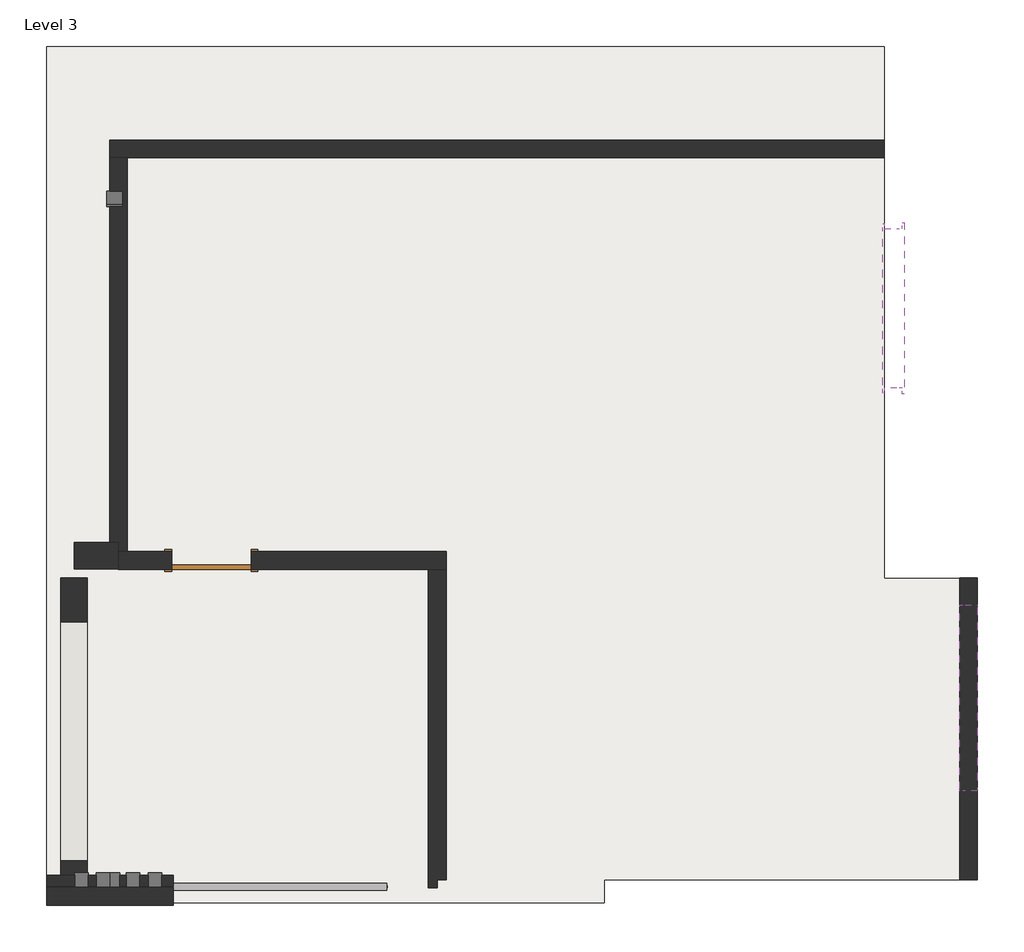
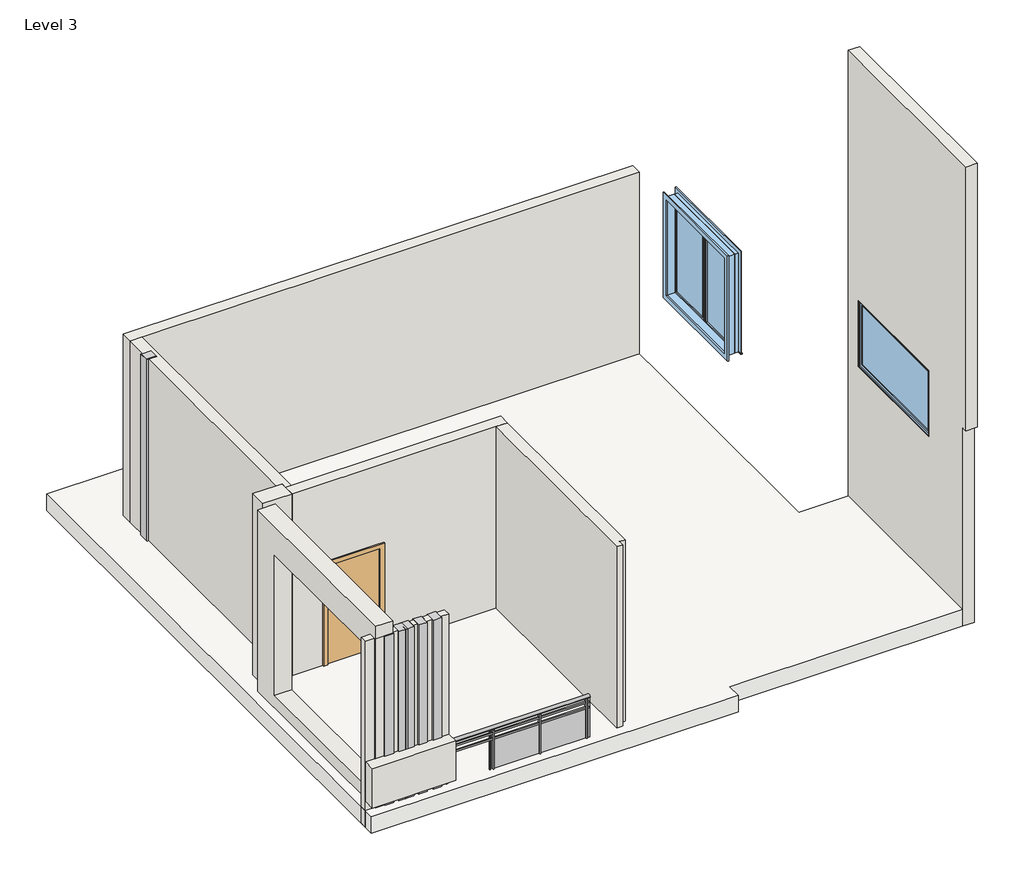
# One storey: 9 walls, 7 proxies, 2 windows, 1 door, 1 railing, 1 roof.
"""IFC4 building model written with IfcOpenShell, lengths in millimetres."""

from ifc_helpers import new_model, si_unit, point, frame, origin, place, context, project, spatial, polyline, ellipse_curve, trimmed, outline, extrude, faceted_brep, transform, mapped, element, save
from ifc_brep_helpers import plane_surface, extruded_surface, advanced_brep
from components import door_54dd4da4, window_b085ff8d, window_a973ac2f

model = new_model("IFC4")

# Units and contexts
model_context = context("Model", 3, world=origin())
ifc_project = project(units=[si_unit("LENGTHUNIT", "METRE", prefix="MILLI")], contexts=[model_context])

# Site, building, storey
site = spatial("IfcSite", under=ifc_project)
building = spatial("IfcBuilding", under=site)
storey = spatial("IfcBuildingStorey", under=building, Name="Level 3", Elevation=7315.2)

# Proxies
placement = place(None, origin())
element("IfcBuildingElementProxy", 1, Name="Reveal", ObjectType="Reveal", at=placement, inside=storey, context=model_context, shape_type="SweptSolid", body=[
    extrude(outline(polyline([(-10512.8512689, 1545.5272776), (-10512.8512689, 1728.4072776), (-10360.4512689, 1728.4072776), (-10360.4512689, 1545.5272776), (-10512.8512689, 1545.5272776)])), frame((0.0, 0.0, 7315.2), z_axis=(0.0, 0.0, 1.0), x_axis=(1.0, 0.0, 0.0)), (0.0, 0.0, 1.0), 3429.0),
])
element("IfcBuildingElementProxy", 2, Name="Reveal", ObjectType="Reveal", at=placement, inside=storey, context=model_context, shape_type="SweptSolid", body=[
    extrude(outline(polyline([(-10265.2012689, 1545.5272776), (-10265.2012689, 1728.4072776), (-10112.8012689, 1728.4072776), (-10112.8012689, 1545.5272776), (-10265.2012689, 1545.5272776)])), frame((0.0, 0.0, 7315.2), z_axis=(0.0, 0.0, 1.0), x_axis=(1.0, 0.0, 0.0)), (0.0, 0.0, 1.0), 3429.0),
])
element("IfcBuildingElementProxy", 3, Name="Reveal", ObjectType="Reveal", at=placement, inside=storey, context=model_context, shape_type="SweptSolid", body=[
    extrude(outline(polyline([(-10144.6621198, 9556.80098), (-9961.7821198, 9556.80098), (-9961.7821198, 9404.40098), (-10144.6621198, 9404.40098), (-10144.6621198, 9556.80098)])), frame((0.0, 0.0, 7315.2), z_axis=(0.0, 0.0, 1.0), x_axis=(1.0, 0.0, 0.0)), (0.0, 0.0, 1.0), 3657.6),
])
element("IfcBuildingElementProxy", 4, Name="Reveal", ObjectType="Reveal", at=placement, inside=storey, context=model_context, shape_type="SweptSolid", body=[
    extrude(outline(polyline([(-10144.6621198, 9531.40098), (-9961.7821198, 9531.40098), (-9961.7821198, 9379.00098), (-10144.6621198, 9379.00098), (-10144.6621198, 9531.40098)])), frame((0.0, 0.0, 7315.2), z_axis=(0.0, 0.0, 1.0), x_axis=(1.0, 0.0, 0.0)), (0.0, 0.0, 1.0), 3657.6),
])
element("IfcBuildingElementProxy", 5, Name="Reveal", ObjectType="Reveal", at=placement, inside=storey, context=model_context, shape_type="SweptSolid", body=[
    extrude(outline(polyline([(-9668.3012689, 1545.5272776), (-9668.3012689, 1728.4072776), (-9515.9012689, 1728.4072776), (-9515.9012689, 1545.5272776), (-9668.3012689, 1545.5272776)])), frame((0.0, 0.0, 7315.2), z_axis=(0.0, 0.0, 1.0), x_axis=(1.0, 0.0, 0.0)), (0.0, 0.0, 1.0), 3429.0),
])
element("IfcBuildingElementProxy", 6, Name="Reveal", ObjectType="Reveal", at=placement, inside=storey, context=model_context, shape_type="SweptSolid", body=[
    extrude(outline(polyline([(-9922.3012689, 1545.5272776), (-9922.3012689, 1728.4072776), (-9769.9012689, 1728.4072776), (-9769.9012689, 1545.5272776), (-9922.3012689, 1545.5272776)])), frame((0.0, 0.0, 7315.2), z_axis=(0.0, 0.0, 1.0), x_axis=(1.0, 0.0, 0.0)), (0.0, 0.0, 1.0), 3429.0),
])
element("IfcBuildingElementProxy", 7, Name="Reveal", ObjectType="Reveal", at=placement, inside=storey, context=model_context, shape_type="SweptSolid", body=[
    extrude(outline(polyline([(-10150.9012689, 1545.5272776), (-10150.9012689, 1728.4072776), (-9998.5012689, 1728.4072776), (-9998.5012689, 1545.5272776), (-10150.9012689, 1545.5272776)])), frame((0.0, 0.0, 7315.2), z_axis=(0.0, 0.0, 1.0), x_axis=(1.0, 0.0, 0.0)), (0.0, 0.0, 1.0), 3429.0),
])

# Door
door_shape = door_54dd4da4(model_context)
element("IfcDoor", 8, ObjectType="Single-Flush : 36\" x 84\"", at=placement, inside=storey, context=model_context, shape_type="MappedRepresentation", body=[
    mapped(door_shape, transform((-8945.7821198, 5315.00098, 7315.2), x_axis=(-1.0, 0.0, 0.0), y_axis=(0.0, -1.0, 0.0), z_axis=(0.0, 0.0, 1.0))),
])

# Railing
element("IfcRailing", 9, ObjectType="Glass Panel - Bottom Fill", at=placement, inside=storey, context=model_context, shape_type="SolidModel", body=[
    advanced_brep(
    [(-9425.1307892, 1607.7572776, 8382.0), (-9425.1307892, 1531.5572776, 8382.0), (-6935.9307892, 1607.7572776, 8382.0), (-6935.9307892, 1531.5572776, 8382.0)],
    [
        (0, 1, ellipse_curve(frame((-9425.1307892, 1569.6572776, 8382.0), z_axis=(-1.0, 0.0, 0.0), x_axis=(0.0, -1.0, 0.0)), 38.1, 28.575)),
        (1, 0, ellipse_curve(frame((-9425.1307892, 1569.6572776, 8382.0), z_axis=(-1.0, 0.0, 0.0), x_axis=(0.0, -1.0, 0.0)), 38.1, 28.575)),
        (2, 3, ellipse_curve(frame((-6935.9307892, 1569.6572776, 8382.0), z_axis=(1.0, 0.0, 0.0), x_axis=(0.0, -1.0, 0.0)), 38.1, 28.575)),
        (3, 2, ellipse_curve(frame((-6935.9307892, 1569.6572776, 8382.0), z_axis=(1.0, 0.0, 0.0), x_axis=(0.0, -1.0, 0.0)), 38.1, 28.575)),
        (0, 2),
        (3, 1),
    ],
    [
        plane_surface(frame((-9425.1307892, 1569.6572776, 8382.0), z_axis=(-1.0, 0.0, 0.0), x_axis=(0.0, 1.0, 0.0))),
        plane_surface(frame((-6935.9307892, 1569.6572776, 8382.0), z_axis=(1.0, 0.0, 0.0), x_axis=(0.0, 1.0, 0.0))),
        extruded_surface(trimmed(ellipse_curve(frame((-6935.9307892, 1569.6572776, 8382.0), z_axis=(-1.0, 0.0, 0.0), x_axis=(0.0, -1.0, 0.0)), 38.1, 28.575), [point((-6935.9307892, 1607.7572776, 8382.0))], [point((-6935.9307892, 1531.5572776, 8382.0))], True, "CARTESIAN"), (-2489.2000000000007, 0.0, 0.0), 2489.2000000000007),
        extruded_surface(trimmed(ellipse_curve(frame((-6935.9307892, 1569.6572776, 8382.0), z_axis=(-1.0, 0.0, 0.0), x_axis=(0.0, -1.0, 0.0)), 38.1, 28.575), [point((-6935.9307892, 1531.5572776, 8382.0))], [point((-6935.9307892, 1607.7572776, 8382.0))], True, "CARTESIAN"), (-2489.2000000000007, 0.0, 0.0), 2489.2000000000007),
    ],
    [
        (0, [[1, 2]]),
        (1, [[3, 4]]),
        (2, [[-1, 5, -4, 6]]),
        (3, [[-2, -6, -3, -5]]),
    ],
),
    extrude(outline(polyline([(-9425.1307892, 1556.9572776), (-9425.1307892, 1582.3572776), (-6935.9307892, 1582.3572776), (-6935.9307892, 1556.9572776), (-9425.1307892, 1556.9572776)])), frame((0.0, 0.0, 8267.7), z_axis=(0.0, 0.0, 1.0), x_axis=(1.0, 0.0, 0.0)), (0.0, 0.0, 1.0), 25.4),
    extrude(outline(polyline([(-9425.1307892, 1556.9572776), (-9425.1307892, 1582.3572776), (-6935.9307892, 1582.3572776), (-6935.9307892, 1556.9572776), (-9425.1307892, 1556.9572776)])), frame((0.0, 0.0, 8166.1), z_axis=(0.0, 0.0, 1.0), x_axis=(1.0, 0.0, 0.0)), (0.0, 0.0, 1.0), 25.4),
    extrude(outline(polyline([(-6993.0807892, 1544.2572776), (-6993.0807892, 1595.0572776), (-6980.3807892, 1595.0572776), (-6980.3807892, 1544.2572776), (-6993.0807892, 1544.2572776)])), frame((0.0, 0.0, 7467.6), z_axis=(0.0, 0.0, 1.0), x_axis=(1.0, 0.0, 0.0)), (0.0, 0.0, 1.0), 885.6788223),
    extrude(outline(polyline([(-7799.5307892, 1576.1924346), (-6986.7307892, 1576.1924346), (-6986.7307892, 1569.8424346), (-7799.5307892, 1569.8424346), (-7799.5307892, 1576.1924346)])), frame((0.0, 0.0, 7569.2), z_axis=(0.0, 0.0, 1.0), x_axis=(1.0, 0.0, 0.0)), (0.0, 0.0, 1.0), 596.9),
    extrude(outline(polyline([(-7805.8807892, 1544.2572776), (-7805.8807892, 1595.0572776), (-7793.1807892, 1595.0572776), (-7793.1807892, 1544.2572776), (-7805.8807892, 1544.2572776)])), frame((0.0, 0.0, 7467.6), z_axis=(0.0, 0.0, 1.0), x_axis=(1.0, 0.0, 0.0)), (0.0, 0.0, 1.0), 885.6788223),
    extrude(outline(polyline([(-8612.3307892, 1576.1924346), (-7799.5307892, 1576.1924346), (-7799.5307892, 1569.8424346), (-8612.3307892, 1569.8424346), (-8612.3307892, 1576.1924346)])), frame((0.0, 0.0, 7569.2), z_axis=(0.0, 0.0, 1.0), x_axis=(1.0, 0.0, 0.0)), (0.0, 0.0, 1.0), 596.9),
    extrude(outline(polyline([(-8618.6807892, 1544.2572776), (-8618.6807892, 1595.0572776), (-8605.9807892, 1595.0572776), (-8605.9807892, 1544.2572776), (-8618.6807892, 1544.2572776)])), frame((0.0, 0.0, 7467.6), z_axis=(0.0, 0.0, 1.0), x_axis=(1.0, 0.0, 0.0)), (0.0, 0.0, 1.0), 885.6788223),
    extrude(outline(polyline([(-8672.6557892, 1560.1322776), (-8672.6557892, 1579.1822776), (-8653.6057892, 1579.1822776), (-8653.6057892, 1560.1322776), (-8672.6557892, 1560.1322776)])), frame((0.0, 0.0, 7467.6), z_axis=(0.0, 0.0, 1.0), x_axis=(1.0, 0.0, 0.0)), (0.0, 0.0, 1.0), 885.6788223),
    extrude(outline(polyline([(-6948.6307892, 1560.1322776), (-6948.6307892, 1579.1822776), (-6929.5807892, 1579.1822776), (-6929.5807892, 1560.1322776), (-6948.6307892, 1560.1322776)])), frame((0.0, 0.0, 7467.6), z_axis=(0.0, 0.0, 1.0), x_axis=(1.0, 0.0, 0.0)), (0.0, 0.0, 1.0), 885.6788223),
    extrude(outline(polyline([(-9431.4807892, 1560.1322776), (-9431.4807892, 1579.1822776), (-9412.4307892, 1579.1822776), (-9412.4307892, 1560.1322776), (-9431.4807892, 1560.1322776)])), frame((0.0, 0.0, 7467.6), z_axis=(0.0, 0.0, 1.0), x_axis=(1.0, 0.0, 0.0)), (0.0, 0.0, 1.0), 885.6788223),
])

# Roof
element("IfcRoof", 10, ObjectType="Generic - 12\"", at=placement, inside=storey, context=model_context, shape_type="SweptSolid", body=[
    extrude(outline(polyline([(-10836.7012689, 11214.3911137), (-1224.1821198, 11214.3911137), (-1224.1821198, 5111.80098), (-360.5821198, 5111.80098), (-360.5821198, 1650.6780349), (-4435.9012689, 1650.6780349), (-4435.9012689, 1387.3881635), (-10836.7012689, 1387.3881635), (-10836.7012689, 11214.3911137)])), frame((0.0, 0.0, 7315.2), z_axis=(0.0, 0.0, 1.0), x_axis=(1.0, 0.0, 0.0)), (0.0, 0.0, 1.0), 304.8),
])

# Walls
element("IfcWall", 11, ObjectType="Generic - 12\"", at=placement, inside=storey, context=model_context, shape_type="SweptSolid", body=[
    extrude(outline(polyline([(1558.4652184, 7315.2), (1558.4652184, 7797.8), (1563.3072776, 7797.8), (1563.3072776, 10744.2), (1558.4652184, 10744.2), (1558.4652184, 10972.8), (5114.4652184, 10972.8), (5114.4652184, 7315.2), (1558.4652184, 7315.2)]), holes=[polyline([(1866.5256437, 10440.4581243), (1866.5256437, 7849.6581243), (4609.7256437, 7849.6581243), (4609.7256437, 10440.4581243), (1866.5256437, 10440.4581243)])]), frame((-10672.9932957, 0.0, 0.0), z_axis=(1.0, 0.0, 0.0), x_axis=(0.0, 1.0, 0.0)), (0.0, 0.0, 1.0), 304.8),
])
element("IfcWall", 12, ObjectType="Generic - 12\"", at=placement, inside=storey, context=model_context, shape_type="Brep", body=[
    faceted_brep([(-10520.5932957, 5216.0652184, 7315.2), (-10012.5821198, 5216.0652184, 7315.2), (-10012.5821198, 5216.0652184, 10972.8), (-10520.5932957, 5216.0652184, 10972.8), (-10520.5932957, 5520.8652184, 7315.2), (-10520.5932957, 5520.8652184, 10972.8), (-10114.1821198, 5520.8652184, 10972.8), (-10012.5821198, 5520.8652184, 10972.8), (-10012.5821198, 5520.8652184, 7315.2), (-10114.1821198, 5520.8652184, 7315.2), (-10012.5821198, 5416.60098, 7315.2), (-10012.5821198, 5416.60098, 10972.8)], [[[0, 1, 2, 3]], [[4, 5, 6, 7, 8, 9]], [[1, 0, 4, 9, 8, 10]], [[2, 1, 10, 8, 7, 11]], [[3, 2, 11, 7, 6, 5]], [[0, 3, 5, 4]]]),
])
element("IfcWall", 13, ObjectType="Generic - 5\"", at=placement, inside=storey, context=model_context, shape_type="SweptSolid", body=[
    extrude(outline(polyline([(-9383.0024679, 1703.0072776), (-9383.0024679, 1576.0072776), (-9515.9012689, 1576.0072776), (-9515.9012689, 1703.0072776), (-9383.0024679, 1703.0072776)])), frame((0.0, 0.0, 7315.2), z_axis=(0.0, 0.0, 1.0), x_axis=(1.0, 0.0, 0.0)), (0.0, 0.0, 1.0), 3429.0),
    extrude(outline(polyline([(-10836.7012689, 1576.0072776), (-10836.7012689, 1703.0072776), (-10512.8512689, 1703.0072776), (-10512.8512689, 1576.0072776), (-10836.7012689, 1576.0072776)])), frame((0.0, 0.0, 7315.2), z_axis=(0.0, 0.0, 1.0), x_axis=(1.0, 0.0, 0.0)), (0.0, 0.0, 1.0), 3429.0),
    extrude(outline(polyline([(-10360.4512689, 1576.0072776), (-10360.4512689, 1703.0072776), (-10265.2012689, 1703.0072776), (-10265.2012689, 1576.0072776), (-10360.4512689, 1576.0072776)])), frame((0.0, 0.0, 7315.2), z_axis=(0.0, 0.0, 1.0), x_axis=(1.0, 0.0, 0.0)), (0.0, 0.0, 1.0), 3429.0),
    extrude(outline(polyline([(-9668.3012689, 1703.0072776), (-9668.3012689, 1576.0072776), (-9769.9012689, 1576.0072776), (-9769.9012689, 1703.0072776), (-9668.3012689, 1703.0072776)])), frame((0.0, 0.0, 7315.2), z_axis=(0.0, 0.0, 1.0), x_axis=(1.0, 0.0, 0.0)), (0.0, 0.0, 1.0), 3429.0),
    extrude(outline(polyline([(-9922.3012689, 1703.0072776), (-9922.3012689, 1576.0072776), (-9998.5012689, 1576.0072776), (-9998.5012689, 1703.0072776), (-9922.3012689, 1703.0072776)])), frame((0.0, 0.0, 7315.2), z_axis=(0.0, 0.0, 1.0), x_axis=(1.0, 0.0, 0.0)), (0.0, 0.0, 1.0), 3429.0),
])
element("IfcWall", 14, ObjectType="Generic - 8\"", at=placement, inside=storey, context=model_context, shape_type="Brep", body=[
    faceted_brep([(-10114.1821198, 9937.80098, 7315.2), (-9910.9821198, 9937.80098, 7315.2), (-1224.1821198, 9937.80098, 7315.2), (-1224.1821198, 9937.80098, 10972.8), (-9910.9821198, 9937.80098, 10972.8), (-10114.1821198, 9937.80098, 10972.8), (-10114.1821198, 10141.00098, 7315.2), (-10114.1821198, 10141.00098, 10972.8), (-1224.1821198, 10141.00098, 10972.8), (-1224.1821198, 10141.00098, 7315.2)], [[[0, 1, 2, 3, 4, 5]], [[6, 7, 8, 9]], [[2, 1, 0, 6, 9]], [[5, 4, 3, 8, 7]], [[0, 5, 7, 6]], [[3, 2, 9, 8]]]),
])
element("IfcWall", 15, ObjectType="Generic - 8\"", at=placement, inside=storey, context=model_context, shape_type="SweptSolid", body=[
    extrude(outline(polyline([(-9910.9821198, 9937.80098), (-9910.9821198, 5416.60098), (-10012.5821198, 5416.60098), (-10012.5821198, 5520.8652184), (-10114.1821198, 5520.8652184), (-10114.1821198, 9379.00098), (-9961.7821198, 9379.00098), (-9961.7821198, 9556.80098), (-10114.1821198, 9556.80098), (-10114.1821198, 9937.80098), (-9910.9821198, 9937.80098)])), frame((0.0, 0.0, 7315.2), z_axis=(0.0, 0.0, 1.0), x_axis=(1.0, 0.0, 0.0)), (0.0, 0.0, 1.0), 3657.6),
])
element("IfcWall", 16, ObjectType="Generic - 8\"", at=placement, inside=storey, context=model_context, shape_type="SweptSolid", body=[
    extrude(outline(polyline([(1558.4652184, 15849.6), (5111.80098, 15849.6), (5111.80098, 7315.2), (4857.80098, 7315.2), (4857.80098, 7475.8655485), (2724.20098, 7475.8655485), (2724.20098, 7315.2), (1650.6780349, 7315.2), (1650.6780349, 10972.8), (1558.4652184, 10972.8), (1558.4652184, 15849.6)]), holes=[polyline([(4807.00098, 11414.8102851), (2673.40098, 11414.8102851), (2673.40098, 10195.6102851), (4807.00098, 10195.6102851), (4807.00098, 11414.8102851)])]), frame((-360.5821198, 0.0, 0.0), z_axis=(1.0, 0.0, 0.0), x_axis=(0.0, 1.0, 0.0)), (0.0, 0.0, 1.0), 203.2),
])
element("IfcWall", 17, ObjectType="Generic - 8\"", at=placement, inside=storey, context=model_context, shape_type="Brep", body=[
    faceted_brep([(-10012.5821198, 5213.40098, 7315.2), (-9402.9821198, 5213.40098, 7315.2), (-9402.9821198, 5213.40098, 9448.8), (-8488.5821198, 5213.40098, 9448.8), (-8488.5821198, 5213.40098, 7315.2), (-6456.5821198, 5213.40098, 7315.2), (-6253.3821198, 5213.40098, 7315.2), (-6253.3821198, 5213.40098, 10972.8), (-6456.5821198, 5213.40098, 10972.8), (-10012.5821198, 5213.40098, 10972.8), (-9402.9821198, 5416.60098, 9448.8), (-9402.9821198, 5416.60098, 7315.2), (-9910.9821198, 5416.60098, 7315.2), (-10012.5821198, 5416.60098, 7315.2), (-10012.5821198, 5416.60098, 10972.8), (-9910.9821198, 5416.60098, 10972.8), (-6253.3821198, 5416.60098, 10972.8), (-6253.3821198, 5416.60098, 7315.2), (-8488.5821198, 5416.60098, 7315.2), (-8488.5821198, 5416.60098, 9448.8), (-10012.5821198, 5216.0652184, 7315.2), (-10012.5821198, 5216.0652184, 10972.8)], [[[0, 1, 2, 3, 4, 5, 6, 7, 8, 9]], [[10, 11, 12, 13, 14, 15, 16, 17, 18, 19]], [[18, 17, 6, 5, 4]], [[13, 12, 11, 1, 0, 20]], [[9, 8, 7, 16, 15, 14, 21]], [[0, 9, 21, 14, 13, 20]], [[7, 6, 17, 16]], [[2, 1, 11, 10]], [[3, 2, 10, 19]], [[4, 3, 19, 18]]]),
])
element("IfcWall", 18, ObjectType="Generic - 8\"", at=placement, inside=storey, context=model_context, shape_type="SweptSolid", body=[
    extrude(outline(polyline([(-6456.5821198, 1558.4652184), (-6456.5821198, 5213.40098), (-6253.3821198, 5213.40098), (-6253.3821198, 1650.6780349), (-6354.9821198, 1650.6780349), (-6354.9821198, 1558.4652184), (-6456.5821198, 1558.4652184)])), frame((0.0, 0.0, 7315.2), z_axis=(0.0, 0.0, 1.0), x_axis=(1.0, 0.0, 0.0)), (0.0, 0.0, 1.0), 3657.6),
])
element("IfcWall", 19, ObjectType="Generic - 8\"", at=placement, inside=storey, context=model_context, shape_type="Brep", body=[
    faceted_brep([(-10836.7012689, 1360.1072776, 7797.8), (-9383.0024679, 1360.1072776, 7797.8), (-9383.0024679, 1360.1072776, 8527.1638259), (-10836.7012689, 1360.1072776, 8527.1638259), (-10836.7012689, 1563.3072776, 7797.8), (-10836.7012689, 1563.3072776, 8527.1638259), (-9383.0024679, 1563.3072776, 8527.1638259), (-9383.0024679, 1563.3072776, 7797.8), (-10368.1932957, 1563.3072776, 7797.8), (-10672.9932957, 1563.3072776, 7797.8)], [[[0, 1, 2, 3]], [[4, 5, 6, 7, 8, 9]], [[1, 0, 4, 9, 8, 7]], [[2, 1, 7, 6]], [[3, 2, 6, 5]], [[0, 3, 5, 4]]]),
])

# Windows
window_shape = window_b085ff8d(model_context)
element("IfcWindow", 20, ObjectType="Casement Dbl with Trim : 72\" x 36\"", at=placement, inside=storey, context=model_context, shape_type="MappedRepresentation", body=[
    mapped(window_shape, transform((-1141.6321198, 8210.60098, 7964.3075998), x_axis=(0.0, -1.0, 0.0), y_axis=(1.0, 0.0, 0.0), z_axis=(0.0, 0.0, 1.0))),
])
window_2_shape = window_a973ac2f(model_context)
element("IfcWindow", 21, ObjectType="Fixed : 36\" x 72\"", at=placement, inside=storey, context=model_context, shape_type="MappedRepresentation", body=[
    mapped(window_2_shape, transform((-258.9821198, 3778.30098, 9890.8102851), x_axis=(0.0, 1.0, 0.0), y_axis=(-1.0, 0.0, 0.0), z_axis=(0.0, 0.0, 1.0))),
])

save(model, "model.ifc")

# Revit data of these elements
# Type "Single-Flush : 36\" x 84\""
#   Type Mark = "1"
#   Construction Type Id = "MDOOR"
#   Assembly Code = "C1020"
#   Analytic Construction = "Metal"
#   Thickness = 0' - 2"
#   Heat Transfer Coefficient (U) = 0.651978 BTU/(h·ft²·°F)
#   Height = 7' - 0"
#   Trim Projection Ext = 0' - 1"
#   Trim Projection Int = 0' - 1"
#   Trim Width = 0' - 3"
#   Width = 3' - 0"
#   Define Thermal Properties by = 1
#   Door Material = Door - Panel
#   Frame Material = Door - Frame
#   Visual Light Transmittance = 0
#   Solar Heat Gain Coefficient = 0
#   Function = (empty or 0)
#   Wall Closure = (empty or 0)
# Type "Glass Panel - Bottom Fill"
#   Assembly Code = "C2010400"
#   built-in parameter 1008612 = 0.0416667 (stored number, unit not read)
#   built-in parameter 1008611 = 0.0416667 (stored number, unit not read)
#   built-in parameter 1008609 = 0.333333 (stored number, unit not read)
#   built-in parameter 1008604 = 0.166667 (stored number, unit not read)
#   built-in parameter 1008603 = 0.166667 (stored number, unit not read)
#   Railing Height = 3' - 0"
#   built-in parameter 1008630 = 2
#   built-in parameter 1008610 = 2
#   built-in parameter 1008618 = Baluster - Square : 3/4"
# Type "Generic - 12\""
#   Assembly Code = "B1020"
#   Layers, outside or top first: 1' - 0" no material (function 1)
# Type "Generic - 12\""
#   Assembly Code = "B2010"
#   Layers, outside or top first: 1' - 0" no material (function 1)
# Type "Generic - 5\""
#   Assembly Code = "B2010"
#   Layers, outside or top first: 0' - 5" no material (function 1)
# Type "Generic - 8\""
#   Assembly Code = "B2010"
#   Layers, outside or top first: 0' - 8" no material (function 1)
# Type "Casement Dbl with Trim : 72\" x 36\""
#   Type Mark = "11"
#   Construction Type Id = "GSP4R"
#   Assembly Code = "B2020100"
#   Analytic Construction = "1/8 in Pilkington single glazing"
#   Visual Light Transmittance = 0.9
#   Solar Heat Gain Coefficient = 0.78
#   Heat Transfer Coefficient (U) = 0.6496 BTU/(h·ft²·°F)
#   Height = 6' - 0"
#   Default Sill Height = 4' - 0"
#   Trim Projection - Ext. = 0' - 0 1/2"
#   Trim Projection - Int. = 0' - 0 3/4"
#   Trim Width - Exterior = 0' - 3 1/2"
#   Trim Width - Interior = 0' - 3 1/2"
#   Width = 6' - 0"
#   Window Inset = 0' - 0 3/4"
#   Define Thermal Properties by = 1
#   Glass Pane Material = Glass
#   Sash Material = Sash
#   Trim Exterior Material = Trim
#   Trim Interior Material = Trim
#   Wall Closure = (empty or 0)
# Type "Fixed : 36\" x 72\""
#   Type Mark = "9"
#   Construction Type Id = "GSP4R"
#   Assembly Code = "B2020100"
#   Analytic Construction = "1/8 in Pilkington single glazing"
#   Visual Light Transmittance = 0.9
#   Solar Heat Gain Coefficient = 0.78
#   Heat Transfer Coefficient (U) = 0.6496 BTU/(h·ft²·°F)
#   Height = 4' - 0"
#   Default Sill Height = 1' - 0"
#   Width = 7' - 0"
#   Window Inset = 0' - 0 3/4"
#   Define Thermal Properties by = 1
#   Glass Pane Material = Glass
#   Sash Material = Sash
#   Wall Closure = (empty or 0)
# Element 8 (IfcDoor, "Single-Flush : 36\" x 84\"")
#   Phase Created = New Construction
#   Materials on its faces: "Door - Frame", "Door - Panel"
# Element 9 (IfcRailing, "Glass Panel - Bottom Fill")
#   built-in parameter 1008621 = 0.5 (stored number, unit not read)
#   Phase Created = New Construction
#   Materials on its faces: "Glass"
# Element 10 (IfcRoof, "Generic - 12\"")
#   built-in parameter 1001705 = 25 (stored number, unit not read)
#   built-in parameter 1001710 = 33615
#   Phase Created = New Construction
#   Materials on its faces: "Default Roof", "Laminate, Ivory, Matte"
# Elements 11, 12 (IfcWall, "Generic - 12\"")
#   Top Offset = 0' - 0"
#   Base Offset = 0' - 0"
#   Unconnected Height = 12' - 0"
#   wall height = 12' - 0"
#   Phase Created = New Construction
#   Base Constraint = Level 3
#   Materials on its faces: "Default Wall"
# Element 13 (IfcWall, "Generic - 5\"")
#   Top Offset = 0' - 0"
#   Base Offset = 0' - 0"
#   Unconnected Height = 11' - 3"
#   wall height = 11' - 3"
#   Phase Created = New Construction
#   Base Constraint = Level 3
#   Materials on its faces: "Default Wall", "Laminate, Ivory, Matte"
# Elements 14, 15, 17, 18 (IfcWall, "Generic - 8\"")
#   Top Offset = 0' - 0"
#   Base Offset = 0' - 0"
#   Unconnected Height = 12' - 0"
#   wall height = 12' - 0"
#   Phase Created = New Construction
#   Base Constraint = Level 3
#   Materials on its faces: "Default Wall"
# Element 16 (IfcWall, "Generic - 8\"")
#   Top Offset = 0' - 0"
#   Base Offset = 0' - 0"
#   Unconnected Height = 28' - 0"
#   wall height = 28' - 0"
#   Phase Created = New Construction
#   Base Constraint = Level 3
#   Materials on its faces: "Default Wall"
# Element 19 (IfcWall, "Generic - 8\"")
#   built-in parameter 1001111 = 1' - 7"
#   Top Offset = 0' - 0"
#   Base Offset = 1' - 7"
#   Unconnected Height = 2' - 4.71511"
#   wall height = 2' - 4.71511"
#   Phase Created = New Construction
#   Base Constraint = Level 3
#   Materials on its faces: "Default Wall", "Brick, Common"
# Element 20 (IfcWindow, "Casement Dbl with Trim : 72\" x 36\"")
#   Mark = "8"
#   Phase Created = New Construction
#   Materials on its faces: "Sash", "Trim", "Glass"
# Element 21 (IfcWindow, "Fixed : 36\" x 72\"")
#   Mark = "3"
#   Phase Created = New Construction
#   Materials on its faces: "Sash", "Glass"
# Materials
#   "Door - Panel": class "Wood", colour RGB 210 159 95, transparency 0
#   "Door - Frame": colour RGB 118 70 51, transparency 0
#   "Glass": class "Glass", colour RGB 0 128 192, transparency 0.75, Description = "Soda Lime Glass", Cost = 0
#   "Sash": class "Wood", colour RGB 224 178 126, transparency 0
#   "Trim": class "Wood", colour RGB 224 178 126, transparency 0
#   "Default Roof": colour RGB 88 101 114, transparency 0
#   "Laminate, Ivory, Matte": class "Plastic", colour RGB 247 247 239, transparency 0, Description = "Plastic Laminate - Ivory, Matte", Cost = 0
#   "Default Wall": colour RGB 128 128 128, transparency 0
#   "Brick, Common": class "Masonry", colour RGB 170 98 104, transparency 0, Description = "Common brick", Cost = 0
